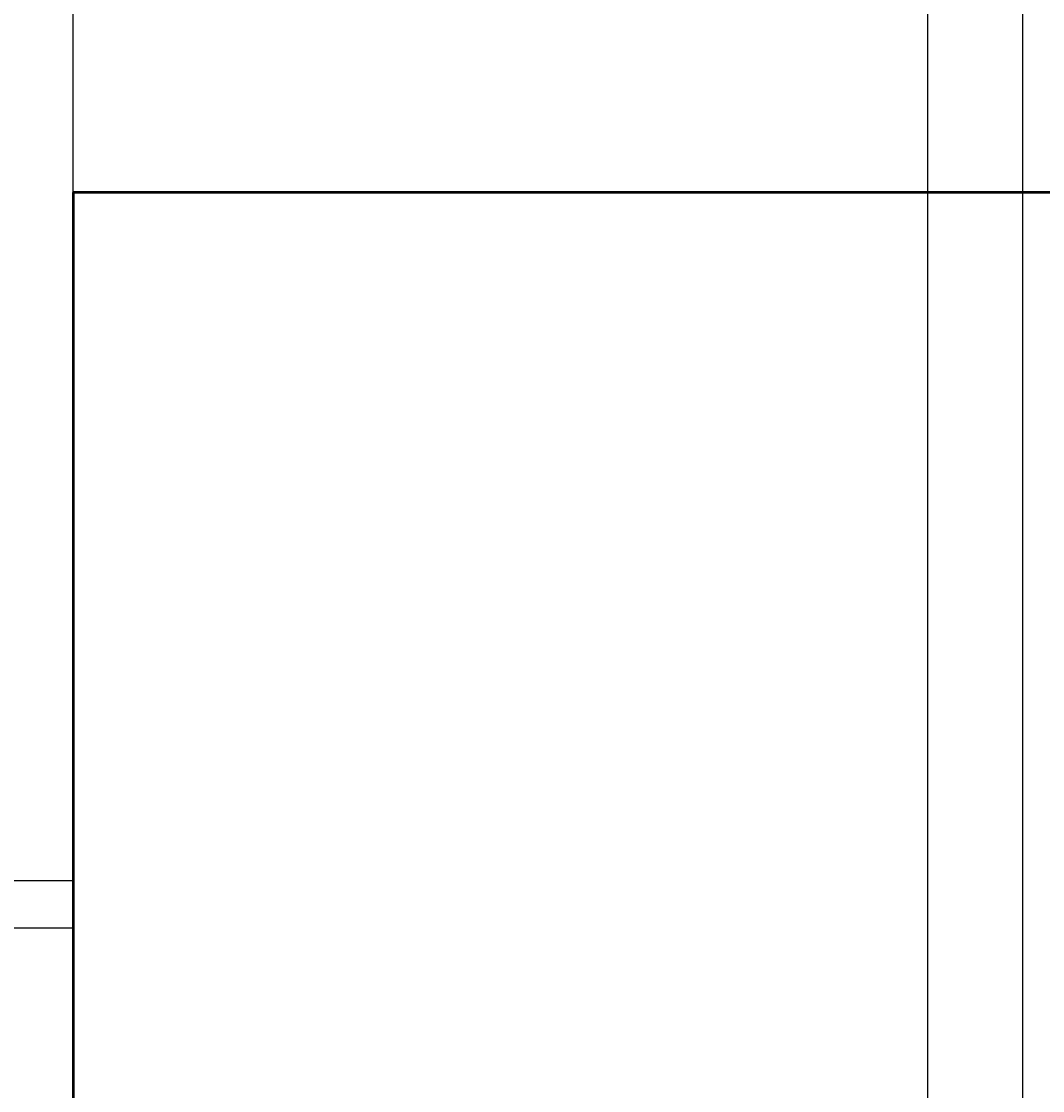
# Model space of a CAD drawing. Units: inches. Extents: x 37 to 824, y -700 to 234.
# Tile 33 of 77: x 168 to 211, y -206 to -161. Entities that reach past the tile are written whole.
import ezdxf

# ---------------------------------------------------------------- set-up
doc = ezdxf.new("R2010")
doc.units = ezdxf.units.IN
doc.header["$MEASUREMENT"] = 0
for name, color, linetype, lineweight in [('A-ANNO-DIMS', 2, 'Continuous', 18), ('A-GLAZ', 4, 'Continuous', 25), ('A-WALL', 2, 'Continuous', 50)]:
    doc.layers.add(name, color=color, linetype=linetype, lineweight=lineweight)
doc.styles.get("Standard").update_dxf_attribs({"font": 'arial.ttf'})
doc.dimstyles.get("Standard").update_dxf_attribs({"dimtxt": 0.18, "dimasz": 0.18, "dimexe": 0.18, "dimexo": 0.0625, "dimgap": 0.09, "dimtad": 0, "dimtih": 1, "dimtoh": 1, "dimdec": 1, "dimzin": 0, "dimdsep": 46, "dimlunit": 4, "dimtxsty": 'Standard', "dimcen": 0.09, "dimadec": 0, "dimazin": 0, "dimtfac": 1, "dimtdec": 1, "dimtofl": 0, "dimtmove": 0, "dimatfit": 3, "dimfxl": 1, "dimtolj": 1, "dimtzin": 0, "dimarcsym": 0})

# ---------------------------------------------------------------- blocks, each defined once
blk = doc.blocks.new('WIN-900')
for p, q in [((0, 9), (0, 0)), ((2, 9), (2, 0)), ((20, 9), (20, 0)), ((38, 9), (38, 0)), ((40, 9), (40, 0)), ((38, 5.5), (2, 5.5)), ((38, 3.5), (2, 3.5))]:
    blk.add_line(p, q)
blk = doc.blocks.new('*D80')
at = {"layer": 'A-ANNO-DIMS', "color": 0, "lineweight": -2, "ltscale": 0.5, "transparency": 16777216}
for p, q in [((170.077, -167.972), (170.077, -400.406)), ((250.19, -167.972), (250.19, -400.406)), ((170.257, -400.226), (209.804, -400.226)), ((250.01, -400.226), (210.463, -400.226))]:
    blk.add_line(p, q, dxfattribs=at)
at = {"layer": 'A-ANNO-DIMS', "color": 0, "ltscale": 0.5, "transparency": 16777216}
for points in [[(170.257, -400.196), (170.257, -400.256), (170.077, -400.226)], [(250.01, -400.196), (250.01, -400.256), (250.19, -400.226)]]:
    blk.add_solid(points, dxfattribs=at)
at = {"layer": 'Defpoints', "color": 0, "ltscale": 0.5, "transparency": 16777216}
for p in [(170.077, -167.91), (250.19, -167.91), (250.19, -400.226)]:
    blk.add_point(p, dxfattribs=at)
at = {"layer": 'A-ANNO-DIMS', "color": 0, "ltscale": 0.5, "transparency": 16777216, "insert": (210.133, -400.226), "char_height": 0.18, "attachment_point": 5}
blk.add_mtext('\\A1;6\'-8"', dxfattribs=at)
blk = doc.blocks.new('*D84')
at = {"layer": 'A-ANNO-DIMS', "color": 0, "lineweight": -2, "ltscale": 0.5, "transparency": 16777216}
for p, q in [((170.077, -265.847), (170.077, 234.17)), ((170.257, 233.99), (189.748, 233.99)), ((209.897, 233.99), (190.406, 233.99)), ((210.077, -265.847), (210.077, 234.17))]:
    blk.add_line(p, q, dxfattribs=at)
at = {"layer": 'A-ANNO-DIMS', "color": 0, "ltscale": 0.5, "transparency": 16777216}
for points in [[(170.257, 234.02), (170.257, 233.96), (170.077, 233.99)], [(209.897, 234.02), (209.897, 233.96), (210.077, 233.99)]]:
    blk.add_solid(points, dxfattribs=at)
at = {"layer": 'Defpoints', "color": 0, "ltscale": 0.5, "transparency": 16777216}
for p in [(210.077, 233.99), (170.077, -265.91), (210.077, -265.91)]:
    blk.add_point(p, dxfattribs=at)
at = {"layer": 'A-ANNO-DIMS', "color": 0, "ltscale": 0.5, "transparency": 16777216, "insert": (190.077, 233.99), "char_height": 0.18, "attachment_point": 5}
blk.add_mtext('\\A1;3\'-4"', dxfattribs=at)
blk = doc.blocks.new('*D85')
at = {"layer": 'A-ANNO-DIMS', "color": 0, "lineweight": -2, "ltscale": 0.5, "transparency": 16777216}
for p, q in [((170.077, -356.847), (170.077, 234.17)), ((170.257, 233.99), (187.748, 233.99)), ((205.897, 233.99), (188.406, 233.99)), ((206.077, -356.847), (206.077, 234.17))]:
    blk.add_line(p, q, dxfattribs=at)
at = {"layer": 'A-ANNO-DIMS', "color": 0, "ltscale": 0.5, "transparency": 16777216}
for points in [[(170.257, 234.02), (170.257, 233.96), (170.077, 233.99)], [(205.897, 234.02), (205.897, 233.96), (206.077, 233.99)]]:
    blk.add_solid(points, dxfattribs=at)
at = {"layer": 'Defpoints', "color": 0, "ltscale": 0.5, "transparency": 16777216}
for p in [(206.077, 233.99), (170.077, -356.91), (206.077, -356.91)]:
    blk.add_point(p, dxfattribs=at)
at = {"layer": 'A-ANNO-DIMS', "color": 0, "ltscale": 0.5, "transparency": 16777216, "insert": (188.077, 233.99), "char_height": 0.18, "attachment_point": 5}
blk.add_mtext('\\A1;3\'-0"', dxfattribs=at)
blk = doc.blocks.new('*D86')
at = {"layer": 'A-ANNO-DIMS', "color": 0, "lineweight": -2, "ltscale": 0.5, "transparency": 16777216}
for p, q in [((206.077, -356.847), (206.077, 234.17)), ((206.257, 233.99), (210.678, 233.99)), ((215.897, 233.99), (211.476, 233.99)), ((216.077, -356.847), (216.077, 234.17))]:
    blk.add_line(p, q, dxfattribs=at)
at = {"layer": 'A-ANNO-DIMS', "color": 0, "ltscale": 0.5, "transparency": 16777216}
for points in [[(206.257, 234.02), (206.257, 233.96), (206.077, 233.99)], [(215.897, 234.02), (215.897, 233.96), (216.077, 233.99)]]:
    blk.add_solid(points, dxfattribs=at)
at = {"layer": 'Defpoints', "color": 0, "ltscale": 0.5, "transparency": 16777216}
for p in [(216.077, 233.99), (206.077, -356.91), (216.077, -356.91)]:
    blk.add_point(p, dxfattribs=at)
at = {"layer": 'A-ANNO-DIMS', "color": 0, "ltscale": 0.5, "transparency": 16777216, "insert": (211.077, 233.99), "char_height": 0.18, "attachment_point": 5}
blk.add_mtext('\\A1;0\'-10"', dxfattribs=at)

msp = doc.modelspace()

# ---------------------------------------------------------------- linework, layer by layer
at = {"layer": 'A-WALL'}
for p, q in [((170.077, -167.91), (170.077, -265.91)), ((250.19, -167.91), (170.077, -167.91))]:
    msp.add_line(p, q, dxfattribs=at)

# ---------------------------------------------------------------- block references
at = {"layer": 'A-GLAZ', "rotation": 269.9999999999999}
msp.add_blockref('WIN-900', (161.077, -196.909), dxfattribs=at)

# ---------------------------------------------------------------- dimensions: what is measured, and where the dimension line sits
at = {"layer": 'A-ANNO-DIMS', "ltscale": 0.5}
for base, p1, p2, picture, middle in [((210.077, 233.99), (170.077, -265.91), (210.077, -265.91), '*D84', (190.077, 233.99)), ((206.077, 233.99), (170.077, -356.91), (206.077, -356.91), '*D85', (188.077, 233.99)), ((216.077, 233.99), (206.077, -356.91), (216.077, -356.91), '*D86', (211.077, 233.99)), ((250.19, -400.226), (170.077, -167.91), (250.19, -167.91), '*D80', (210.133, -400.226))]:
    dim = msp.add_linear_dim(base=base, p1=p1, p2=p2, dimstyle='Standard', override={"dimdec": 1, "dimlfac": 1, "dimrnd": 0, "dimzin": 1, "dimdsep": 46, "dimlunit": 4, "dimfrac": 2}, dxfattribs=at)
    dim.commit()
    dim.dimension.update_dxf_attribs({"geometry": picture, "text_midpoint": middle})

doc.saveas('drawing.dxf')
